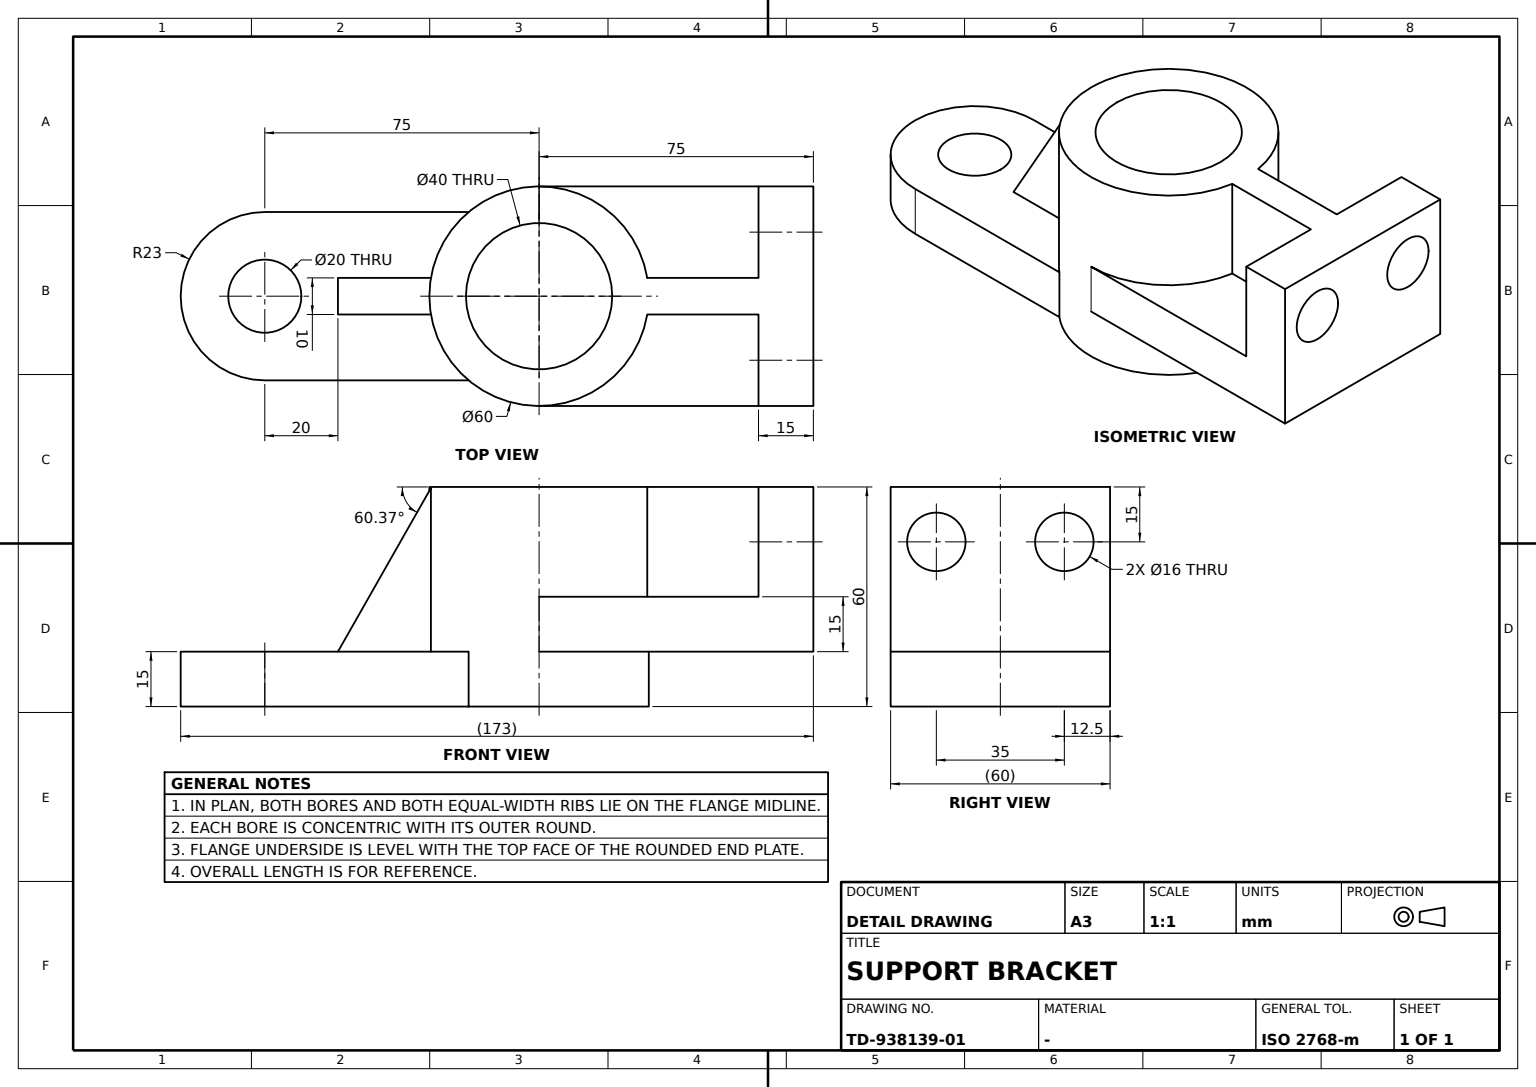
CATIA V5 part; units mm, degrees
ref_plane "Plane1" through (0, 0, 15) normal (0, 0, 1) x (1, 0, 0)
sketch "Sketch1" plane through (0, 0, 0) normal (0, 0, 1) x (1, 0, 0)
  circle A0 centre (0, 0) radius 30
  dimension "radius A0" = 30
extrude "Pad1" add sketch "Sketch1" along normal blind 60
sketch "Sketch2" plane through (0, 0, 60) normal (0, 0, 1) x (1, 0, 0)
  circle A0 centre (0, 0) radius 20
  dimension "radius A0" = 20
extrude "Pocket1" cut sketch "Sketch2" against normal blind 60
sketch "Sketch3" plane through (0, 0, 0) normal (0, 0, -1) x (1, 0, 0)
  line L0 (19.2614, 23) -> (75, 23)
  point P0 (19.2614, 23)
  point P1 (75, 23)
  circle A0 centre (0, 0) radius 30 construction
  line L1 (19.2614, -23) -> (75, -23)
  point P2 (19.2614, -23)
  point P3 (75, -23)
  arc A1 (19.2614, -23) -> (19.2614, 23) centre (0, 0) ccw
  arc A2 (75, 23) -> (75, -23) centre (75, 0) cw
  dimension "distance P1 y axis" = 75
  dimension "distance L0 x axis" = 23
  dimension "distance P3 y axis" = 75
  dimension "distance L1 x axis" = 23
  constraint horizontal L0 x-axis
  constraint horizontal L1 x-axis
  constraint coincidence P0 A0
  constraint coincidence P2 A0
  constraint tangency A2 L1
extrude "Pad2" add sketch "Sketch3" against normal blind 15
sketch "Sketch4" plane through (0, 0, 15) normal (0, 0, 1) x (1, 0, 0)
  circle A0 centre (75, 0) radius 10
  arc A1 (75, -23) -> (75, 23) centre (75, 0) ccw construction
  dimension "radius A0" = 10
  constraint concentricity A0 A1
extrude "Pocket2" cut sketch "Sketch4" against normal blind 15
sketch "Sketch5" plane through (0, 0, 15) normal (0, 0, -1) x (1, 0, 0)
  line L0 (0, 30) -> (-75, 30)
  point P0 (0, 30)
  point P1 (-75, 30)
  circle A0 centre (0, 0) radius 30 construction
  line L1 (0, -30) -> (-75, -30)
  circle A1 centre (0, 0) radius 30 construction
  arc A2 (0, 30) -> (0, -30) centre (0, 0) ccw
  point P2 (0, -30)
  line L2 (-75, 30) -> (-75, -30)
  dimension "distance P1 y axis" = 75
  constraint coincidence P0 y-axis
  constraint coincidence A1 P2
  constraint horizontal L0 x-axis
  constraint horizontal L1 x-axis
  constraint tangency L0 A0
  constraint tangency L1 A0
  constraint vertical L2 y-axis
extrude "Pad3" add sketch "Sketch5" against normal blind 15
sketch "Sketch6" plane through (-75, 0, 0) normal (-1, 0, 0) x (0, -1, 0)
  point P0 (0, 45)
  line L0 (30, 60) -> (30, 30)
  line L1 (30, 30) -> (-30, 30)
  line L2 (-30, 30) -> (-30, 60)
  line L3 (-30, 60) -> (30, 60)
  line L4 (30, 15) -> (30, 30) construction
  line L5 (30, 30) -> (-30, 30) construction
  line L6 (-20, 60) -> (20, 60) construction
  constraint coincidence P0 y-axis
  constraint coincidence L0 L4
  constraint coincidence L1 L5
  constraint coincidence L3 L6
  constraint vertical L0 y-axis
  constraint vertical L2 y-axis
  constraint horizontal L1 x-axis
  constraint horizontal L3 x-axis
  constraint equidistance L0 L2 P0
  constraint equidistance L1 L3 P0
extrude "Pad4" add sketch "Sketch6" against normal blind 15
sketch "Sketch7" plane through (-75, 0, 0) normal (-1, 0, 0) x (0, -1, 0)
  circle A0 centre (-17.5, 45) radius 8
  point P0 (-17.5, 45)
  line L0 (30, 60) -> (-30, 60) construction
  circle A1 centre (17.5, 45) radius 8
  point P1 (17.5, 45)
  dimension "radius A0" = 8
  dimension "distance P0 y axis" = 17.5
  dimension "distance P0 L0" = 15
  dimension "distance P1 L0" = 15
  dimension "distance P1 y axis" = 17.5
  dimension "radius A1" = 8
extrude "Pocket3" cut sketch "Sketch7" against normal blind 15
sketch "Sketch8" plane through (0, 0, 0) normal (0, 1, 0) x (-1, 0, 0)
  line L0 (-29.6086, 59.6424) -> (-55, 15)
  point P0 (-55, 15)
  line L1 (-19.2614, 15) -> (-75, 15) construction
  dimension "distance P0 y axis" = 55
  constraint coincidence P0 L1
rib "Stiffener1" sketch "Sketch8" thickness 10 sides both
sketch "Sketch9" plane through (0, 0, 0) normal (0, 1, 0) x (-1, 0, 0)
  line L0 (29.7952, 60) -> (60, 60)
  point P0 (29.7952, 60)
  point P1 (60, 60)
  line L1 (-30, 60) -> (30, 60) construction
  point P2 (60, 60)
  constraint horizontal L0 x-axis
  constraint coincidence P0 L1
  constraint coincidence P1 P2
rib "Stiffener2" sketch "Sketch9" thickness 10 sides both
